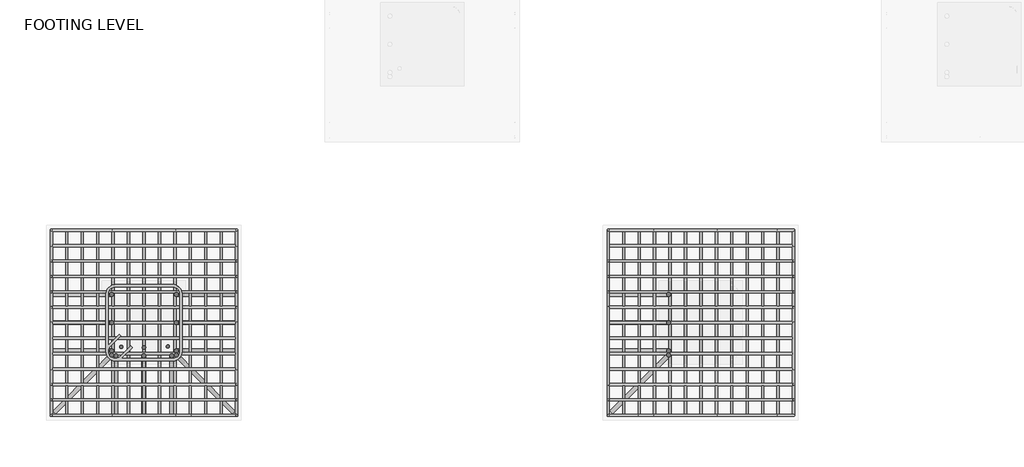
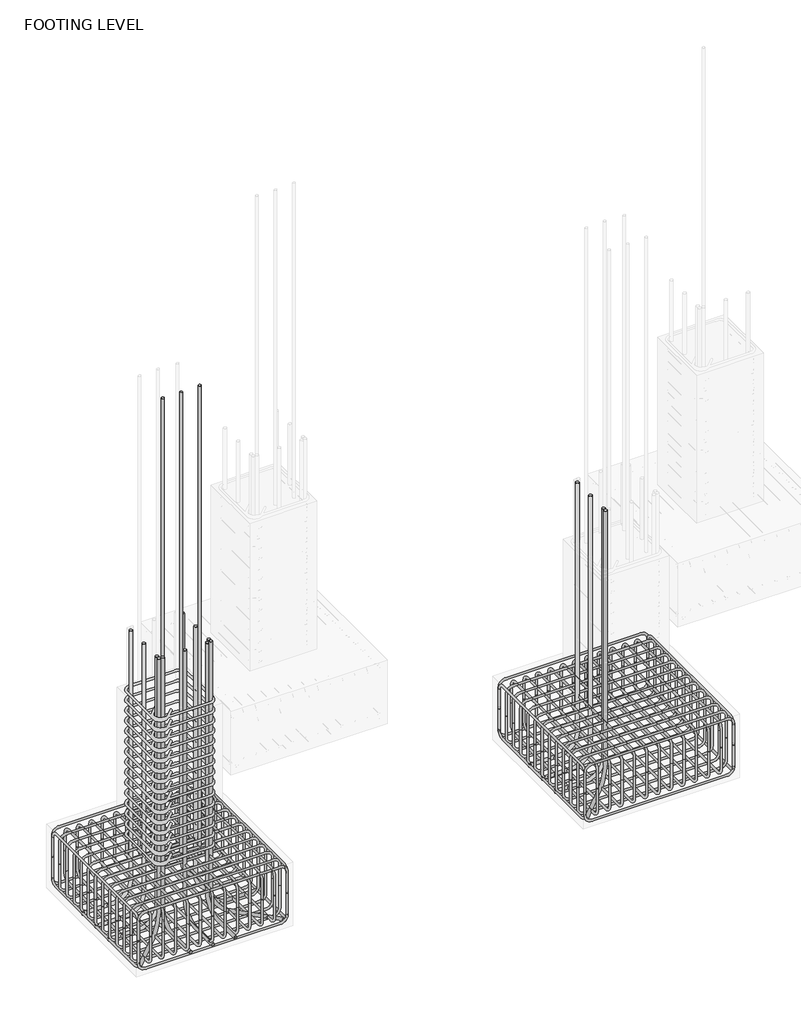
# One storey, part 2 of 10: 20 reinforcing bars.
"""IFC4 building model written with IfcOpenShell, lengths in millimetres."""

from ifc_helpers import new_model, si_unit, point, frame, origin, place, context, project, spatial, polyline, circle_curve, trimmed, segment, composite_curve, source, transform, mapped, element, save
from ifc_brep_helpers import swept_disk

model = new_model("IFC4")

# Units and contexts
model_context = context("Model", 3, world=origin())
ifc_project = project(units=[si_unit("LENGTHUNIT", "METRE", prefix="MILLI")], contexts=[model_context])

# Site, building, storey
site = spatial("IfcSite", under=ifc_project)
building = spatial("IfcBuilding", under=site)
storey = spatial("IfcBuildingStorey", under=building, Name="FOOTING LEVEL", Elevation=-2133.6)

# Reinforcing bars
placement = place(None, origin())
reinforcing_bar_shape = source(origin(), model_context, "Body", "SolidModel", [
    swept_disk(composite_curve([segment(polyline([(-11826.9269037, 756.4829396, -2583.0), (-11826.9269037, 756.4829396, -2905.1)]), True, "CONTINUOUS"), segment(trimmed(circle_curve(frame((-11917.1269037, 756.4829396, -2905.1), z_axis=(0.0, 1.0, 0.0), x_axis=(90.20000000000073, 0.0, 0.0)), 90.2), [point((-11826.9269037, 756.4829396, -2905.1))], [point((-11917.1269037, 756.4829396, -2995.3))], True, "CARTESIAN"), True, "CONTINUOUS"), segment(polyline([(-11917.1269037, 756.4829396, -2995.3), (-13764.9269037, 756.4829396, -2995.3)]), True, "CONTINUOUS"), segment(trimmed(circle_curve(frame((-13764.9269037, 756.4829396, -2905.1), z_axis=(0.0, 1.0, 0.0), x_axis=(0.0, 0.0, -90.20000000000027)), 90.2), [point((-13764.9269037, 756.4829396, -2995.3))], [point((-13855.1269037, 756.4829396, -2905.1))], True, "CARTESIAN"), True, "CONTINUOUS"), segment(polyline([(-13855.1269037, 756.4829396, -2905.1), (-13855.1269037, 756.4829396, -2583.0)]), True, "CONTINUOUS")], self_intersect=False), 12.7),
])
element("IfcReinforcingBar", 1, at=placement, inside=storey, context=model_context, shape_type="MappedRepresentation", body=[
    mapped(reinforcing_bar_shape, transform((0.0, 0.0, 0.0), x_axis=(1.0, 0.0, 0.0), y_axis=(0.0, 1.0, 0.0), z_axis=(0.0, 0.0, 1.0))),
    mapped(reinforcing_bar_shape, transform((0.0, -169.0166667, 0.0), x_axis=(1.0, 0.0, 0.0), y_axis=(0.0, 1.0, 0.0), z_axis=(0.0, 0.0, 1.0))),
    mapped(reinforcing_bar_shape, transform((0.0, -338.0333333, 0.0), x_axis=(1.0, 0.0, 0.0), y_axis=(0.0, 1.0, 0.0), z_axis=(0.0, 0.0, 1.0))),
    mapped(reinforcing_bar_shape, transform((0.0, -507.05, 0.0), x_axis=(1.0, 0.0, 0.0), y_axis=(0.0, 1.0, 0.0), z_axis=(0.0, 0.0, 1.0))),
    mapped(reinforcing_bar_shape, transform((0.0, -676.0666667, 0.0), x_axis=(1.0, 0.0, 0.0), y_axis=(0.0, 1.0, 0.0), z_axis=(0.0, 0.0, 1.0))),
    mapped(reinforcing_bar_shape, transform((0.0, -845.0833333, 0.0), x_axis=(1.0, 0.0, 0.0), y_axis=(0.0, 1.0, 0.0), z_axis=(0.0, 0.0, 1.0))),
    mapped(reinforcing_bar_shape, transform((0.0, -1014.1, 0.0), x_axis=(1.0, 0.0, 0.0), y_axis=(0.0, 1.0, 0.0), z_axis=(0.0, 0.0, 1.0))),
    mapped(reinforcing_bar_shape, transform((0.0, -1183.1166667, 0.0), x_axis=(1.0, 0.0, 0.0), y_axis=(0.0, 1.0, 0.0), z_axis=(0.0, 0.0, 1.0))),
    mapped(reinforcing_bar_shape, transform((0.0, -1352.1333333, 0.0), x_axis=(1.0, 0.0, 0.0), y_axis=(0.0, 1.0, 0.0), z_axis=(0.0, 0.0, 1.0))),
    mapped(reinforcing_bar_shape, transform((0.0, -1521.15, 0.0), x_axis=(1.0, 0.0, 0.0), y_axis=(0.0, 1.0, 0.0), z_axis=(0.0, 0.0, 1.0))),
    mapped(reinforcing_bar_shape, transform((0.0, -1690.1666667, 0.0), x_axis=(1.0, 0.0, 0.0), y_axis=(0.0, 1.0, 0.0), z_axis=(0.0, 0.0, 1.0))),
    mapped(reinforcing_bar_shape, transform((0.0, -1859.1833333, 0.0), x_axis=(1.0, 0.0, 0.0), y_axis=(0.0, 1.0, 0.0), z_axis=(0.0, 0.0, 1.0))),
    mapped(reinforcing_bar_shape, transform((0.0, -2028.2, 0.0), x_axis=(1.0, 0.0, 0.0), y_axis=(0.0, 1.0, 0.0), z_axis=(0.0, 0.0, 1.0))),
])
reinforcing_bar_2_shape = source(origin(), model_context, "Body", "SolidModel", [
    swept_disk(composite_curve([segment(polyline([(-13855.1269037, 756.4829396, -2598.6), (-13855.1269037, 756.4829396, -2276.5)]), True, "CONTINUOUS"), segment(trimmed(circle_curve(frame((-13764.9269037, 756.4829396, -2276.5), z_axis=(0.0, 1.0, 0.0), x_axis=(-90.20000000000073, 0.0, 0.0)), 90.2), [point((-13855.1269037, 756.4829396, -2276.5))], [point((-13764.9269037, 756.4829396, -2186.3))], True, "CARTESIAN"), True, "CONTINUOUS"), segment(polyline([(-13764.9269037, 756.4829396, -2186.3), (-11917.1269037, 756.4829396, -2186.3)]), True, "CONTINUOUS"), segment(trimmed(circle_curve(frame((-11917.1269037, 756.4829396, -2276.5), z_axis=(0.0, 1.0, 0.0), x_axis=(0.0, 0.0, 90.19999999999982)), 90.2), [point((-11917.1269037, 756.4829396, -2186.3))], [point((-11826.9269037, 756.4829396, -2276.5))], True, "CARTESIAN"), True, "CONTINUOUS"), segment(polyline([(-11826.9269037, 756.4829396, -2276.5), (-11826.9269037, 756.4829396, -2598.6)]), True, "CONTINUOUS")], self_intersect=False), 12.7),
])
element("IfcReinforcingBar", 2, at=placement, inside=storey, context=model_context, shape_type="MappedRepresentation", body=[
    mapped(reinforcing_bar_2_shape, transform((0.0, 0.0, 0.0), x_axis=(1.0, 0.0, 0.0), y_axis=(0.0, 1.0, 0.0), z_axis=(0.0, 0.0, 1.0))),
    mapped(reinforcing_bar_2_shape, transform((0.0, -169.0166667, 0.0), x_axis=(1.0, 0.0, 0.0), y_axis=(0.0, 1.0, 0.0), z_axis=(0.0, 0.0, 1.0))),
    mapped(reinforcing_bar_2_shape, transform((0.0, -338.0333333, 0.0), x_axis=(1.0, 0.0, 0.0), y_axis=(0.0, 1.0, 0.0), z_axis=(0.0, 0.0, 1.0))),
    mapped(reinforcing_bar_2_shape, transform((0.0, -507.05, 0.0), x_axis=(1.0, 0.0, 0.0), y_axis=(0.0, 1.0, 0.0), z_axis=(0.0, 0.0, 1.0))),
    mapped(reinforcing_bar_2_shape, transform((0.0, -676.0666667, 0.0), x_axis=(1.0, 0.0, 0.0), y_axis=(0.0, 1.0, 0.0), z_axis=(0.0, 0.0, 1.0))),
    mapped(reinforcing_bar_2_shape, transform((0.0, -845.0833333, 0.0), x_axis=(1.0, 0.0, 0.0), y_axis=(0.0, 1.0, 0.0), z_axis=(0.0, 0.0, 1.0))),
    mapped(reinforcing_bar_2_shape, transform((0.0, -1014.1, 0.0), x_axis=(1.0, 0.0, 0.0), y_axis=(0.0, 1.0, 0.0), z_axis=(0.0, 0.0, 1.0))),
    mapped(reinforcing_bar_2_shape, transform((0.0, -1183.1166667, 0.0), x_axis=(1.0, 0.0, 0.0), y_axis=(0.0, 1.0, 0.0), z_axis=(0.0, 0.0, 1.0))),
    mapped(reinforcing_bar_2_shape, transform((0.0, -1352.1333333, 0.0), x_axis=(1.0, 0.0, 0.0), y_axis=(0.0, 1.0, 0.0), z_axis=(0.0, 0.0, 1.0))),
    mapped(reinforcing_bar_2_shape, transform((0.0, -1521.15, 0.0), x_axis=(1.0, 0.0, 0.0), y_axis=(0.0, 1.0, 0.0), z_axis=(0.0, 0.0, 1.0))),
    mapped(reinforcing_bar_2_shape, transform((0.0, -1690.1666667, 0.0), x_axis=(1.0, 0.0, 0.0), y_axis=(0.0, 1.0, 0.0), z_axis=(0.0, 0.0, 1.0))),
    mapped(reinforcing_bar_2_shape, transform((0.0, -1859.1833333, 0.0), x_axis=(1.0, 0.0, 0.0), y_axis=(0.0, 1.0, 0.0), z_axis=(0.0, 0.0, 1.0))),
    mapped(reinforcing_bar_2_shape, transform((0.0, -2028.2, 0.0), x_axis=(1.0, 0.0, 0.0), y_axis=(0.0, 1.0, 0.0), z_axis=(0.0, 0.0, 1.0))),
])
reinforcing_bar_3_shape = source(origin(), model_context, "Body", "SolidModel", [
    swept_disk(composite_curve([segment(polyline([(-11826.9269037, -1271.7170604, -2559.4978077), (-11826.9269037, -1271.7170604, -2881.5978077)]), True, "CONTINUOUS"), segment(trimmed(circle_curve(frame((-11826.9269037, -1181.5170604, -2881.5978077), z_axis=(1.0, 0.0, 0.0), x_axis=(0.0, -90.20000000000005, 0.0)), 90.2), [point((-11826.9269037, -1271.7170604, -2881.5978077))], [point((-11826.9269037, -1181.5170604, -2971.7978077))], True, "CARTESIAN"), True, "CONTINUOUS"), segment(polyline([(-11826.9269037, -1181.5170604, -2971.7978077), (-11826.9269037, 666.2829396, -2971.7978077)]), True, "CONTINUOUS"), segment(trimmed(circle_curve(frame((-11826.9269037, 666.2829396, -2881.5978077), z_axis=(1.0, 0.0, 0.0), x_axis=(0.0, 0.0, -90.19999999999982)), 90.2), [point((-11826.9269037, 666.2829396, -2971.7978077))], [point((-11826.9269037, 756.4829396, -2881.5978077))], True, "CARTESIAN"), True, "CONTINUOUS"), segment(polyline([(-11826.9269037, 756.4829396, -2881.5978077), (-11826.9269037, 756.4829396, -2559.4978077)]), True, "CONTINUOUS")], self_intersect=False), 12.7),
])
element("IfcReinforcingBar", 3, at=placement, inside=storey, context=model_context, shape_type="MappedRepresentation", body=[
    mapped(reinforcing_bar_3_shape, transform((0.0, 0.0, 0.0), x_axis=(1.0, 0.0, 0.0), y_axis=(0.0, 1.0, 0.0), z_axis=(0.0, 0.0, 1.0))),
    mapped(reinforcing_bar_3_shape, transform((-169.0166667, 0.0, 0.0), x_axis=(1.0, 0.0, 0.0), y_axis=(0.0, 1.0, 0.0), z_axis=(0.0, 0.0, 1.0))),
    mapped(reinforcing_bar_3_shape, transform((-338.0333333, 0.0, 0.0), x_axis=(1.0, 0.0, 0.0), y_axis=(0.0, 1.0, 0.0), z_axis=(0.0, 0.0, 1.0))),
    mapped(reinforcing_bar_3_shape, transform((-507.05, 0.0, 0.0), x_axis=(1.0, 0.0, 0.0), y_axis=(0.0, 1.0, 0.0), z_axis=(0.0, 0.0, 1.0))),
    mapped(reinforcing_bar_3_shape, transform((-676.0666667, 0.0, 0.0), x_axis=(1.0, 0.0, 0.0), y_axis=(0.0, 1.0, 0.0), z_axis=(0.0, 0.0, 1.0))),
    mapped(reinforcing_bar_3_shape, transform((-845.0833333, 0.0, 0.0), x_axis=(1.0, 0.0, 0.0), y_axis=(0.0, 1.0, 0.0), z_axis=(0.0, 0.0, 1.0))),
    mapped(reinforcing_bar_3_shape, transform((-1014.1, 0.0, 0.0), x_axis=(1.0, 0.0, 0.0), y_axis=(0.0, 1.0, 0.0), z_axis=(0.0, 0.0, 1.0))),
    mapped(reinforcing_bar_3_shape, transform((-1183.1166667, 0.0, 0.0), x_axis=(1.0, 0.0, 0.0), y_axis=(0.0, 1.0, 0.0), z_axis=(0.0, 0.0, 1.0))),
    mapped(reinforcing_bar_3_shape, transform((-1352.1333333, 0.0, 0.0), x_axis=(1.0, 0.0, 0.0), y_axis=(0.0, 1.0, 0.0), z_axis=(0.0, 0.0, 1.0))),
    mapped(reinforcing_bar_3_shape, transform((-1521.15, 0.0, 0.0), x_axis=(1.0, 0.0, 0.0), y_axis=(0.0, 1.0, 0.0), z_axis=(0.0, 0.0, 1.0))),
    mapped(reinforcing_bar_3_shape, transform((-1690.1666667, 0.0, 0.0), x_axis=(1.0, 0.0, 0.0), y_axis=(0.0, 1.0, 0.0), z_axis=(0.0, 0.0, 1.0))),
    mapped(reinforcing_bar_3_shape, transform((-1859.1833333, 0.0, 0.0), x_axis=(1.0, 0.0, 0.0), y_axis=(0.0, 1.0, 0.0), z_axis=(0.0, 0.0, 1.0))),
    mapped(reinforcing_bar_3_shape, transform((-2028.2, 0.0, 0.0), x_axis=(1.0, 0.0, 0.0), y_axis=(0.0, 1.0, 0.0), z_axis=(0.0, 0.0, 1.0))),
])
reinforcing_bar_4_shape = source(origin(), model_context, "Body", "SolidModel", [
    swept_disk(composite_curve([segment(polyline([(-13855.1269037, -1271.7170604, -2622.9919875), (-13855.1269037, -1271.7170604, -2300.8919875)]), True, "CONTINUOUS"), segment(trimmed(circle_curve(frame((-13855.1269037, -1181.5170604, -2300.8919875), z_axis=(-1.0, 0.0, 0.0), x_axis=(0.0, -90.20000000000005, 0.0)), 90.2), [point((-13855.1269037, -1271.7170604, -2300.8919875))], [point((-13855.1269037, -1181.5170604, -2210.6919875))], True, "CARTESIAN"), True, "CONTINUOUS"), segment(polyline([(-13855.1269037, -1181.5170604, -2210.6919875), (-13855.1269037, 666.2829396, -2210.6919875)]), True, "CONTINUOUS"), segment(trimmed(circle_curve(frame((-13855.1269037, 666.2829396, -2300.8919875), z_axis=(-1.0, 0.0, 0.0), x_axis=(0.0, 0.0, 90.20000000000027)), 90.2), [point((-13855.1269037, 666.2829396, -2210.6919875))], [point((-13855.1269037, 756.4829396, -2300.8919875))], True, "CARTESIAN"), True, "CONTINUOUS"), segment(polyline([(-13855.1269037, 756.4829396, -2300.8919875), (-13855.1269037, 756.4829396, -2622.9919875)]), True, "CONTINUOUS")], self_intersect=False), 12.7),
])
element("IfcReinforcingBar", 4, at=placement, inside=storey, context=model_context, shape_type="MappedRepresentation", body=[
    mapped(reinforcing_bar_4_shape, transform((0.0, 0.0, 0.0), x_axis=(1.0, 0.0, 0.0), y_axis=(0.0, 1.0, 0.0), z_axis=(0.0, 0.0, 1.0))),
    mapped(reinforcing_bar_4_shape, transform((169.0166667, 0.0, 0.0), x_axis=(1.0, 0.0, 0.0), y_axis=(0.0, 1.0, 0.0), z_axis=(0.0, 0.0, 1.0))),
    mapped(reinforcing_bar_4_shape, transform((338.0333333, 0.0, 0.0), x_axis=(1.0, 0.0, 0.0), y_axis=(0.0, 1.0, 0.0), z_axis=(0.0, 0.0, 1.0))),
    mapped(reinforcing_bar_4_shape, transform((507.05, 0.0, 0.0), x_axis=(1.0, 0.0, 0.0), y_axis=(0.0, 1.0, 0.0), z_axis=(0.0, 0.0, 1.0))),
    mapped(reinforcing_bar_4_shape, transform((676.0666667, 0.0, 0.0), x_axis=(1.0, 0.0, 0.0), y_axis=(0.0, 1.0, 0.0), z_axis=(0.0, 0.0, 1.0))),
    mapped(reinforcing_bar_4_shape, transform((845.0833333, 0.0, 0.0), x_axis=(1.0, 0.0, 0.0), y_axis=(0.0, 1.0, 0.0), z_axis=(0.0, 0.0, 1.0))),
    mapped(reinforcing_bar_4_shape, transform((1014.1, 0.0, 0.0), x_axis=(1.0, 0.0, 0.0), y_axis=(0.0, 1.0, 0.0), z_axis=(0.0, 0.0, 1.0))),
    mapped(reinforcing_bar_4_shape, transform((1183.1166667, 0.0, 0.0), x_axis=(1.0, 0.0, 0.0), y_axis=(0.0, 1.0, 0.0), z_axis=(0.0, 0.0, 1.0))),
    mapped(reinforcing_bar_4_shape, transform((1352.1333333, 0.0, 0.0), x_axis=(1.0, 0.0, 0.0), y_axis=(0.0, 1.0, 0.0), z_axis=(0.0, 0.0, 1.0))),
    mapped(reinforcing_bar_4_shape, transform((1521.15, 0.0, 0.0), x_axis=(1.0, 0.0, 0.0), y_axis=(0.0, 1.0, 0.0), z_axis=(0.0, 0.0, 1.0))),
    mapped(reinforcing_bar_4_shape, transform((1690.1666667, 0.0, 0.0), x_axis=(1.0, 0.0, 0.0), y_axis=(0.0, 1.0, 0.0), z_axis=(0.0, 0.0, 1.0))),
    mapped(reinforcing_bar_4_shape, transform((1859.1833333, 0.0, 0.0), x_axis=(1.0, 0.0, 0.0), y_axis=(0.0, 1.0, 0.0), z_axis=(0.0, 0.0, 1.0))),
    mapped(reinforcing_bar_4_shape, transform((2028.2, 0.0, 0.0), x_axis=(1.0, 0.0, 0.0), y_axis=(0.0, 1.0, 0.0), z_axis=(0.0, 0.0, 1.0))),
])
reinforcing_bar_5_shape = source(origin(), model_context, "Body", "SolidModel", [
    swept_disk(composite_curve([segment(polyline([(-5730.9269037, 756.4829396, -2583.0), (-5730.9269037, 756.4829396, -2905.1)]), True, "CONTINUOUS"), segment(trimmed(circle_curve(frame((-5821.1269037, 756.4829396, -2905.1), z_axis=(0.0, 1.0, 0.0), x_axis=(90.19999999999982, 0.0, 0.0)), 90.2), [point((-5730.9269037, 756.4829396, -2905.1))], [point((-5821.1269037, 756.4829396, -2995.3))], True, "CARTESIAN"), True, "CONTINUOUS"), segment(polyline([(-5821.1269037, 756.4829396, -2995.3), (-7668.9269037, 756.4829396, -2995.3)]), True, "CONTINUOUS"), segment(trimmed(circle_curve(frame((-7668.9269037, 756.4829396, -2905.1), z_axis=(0.0, 1.0, 0.0), x_axis=(0.0, 0.0, -90.20000000000027)), 90.2), [point((-7668.9269037, 756.4829396, -2995.3))], [point((-7759.1269037, 756.4829396, -2905.1))], True, "CARTESIAN"), True, "CONTINUOUS"), segment(polyline([(-7759.1269037, 756.4829396, -2905.1), (-7759.1269037, 756.4829396, -2583.0)]), True, "CONTINUOUS")], self_intersect=False), 12.7),
])
element("IfcReinforcingBar", 5, at=placement, inside=storey, context=model_context, shape_type="MappedRepresentation", body=[
    mapped(reinforcing_bar_5_shape, transform((0.0, 0.0, 0.0), x_axis=(1.0, 0.0, 0.0), y_axis=(0.0, 1.0, 0.0), z_axis=(0.0, 0.0, 1.0))),
    mapped(reinforcing_bar_5_shape, transform((0.0, -169.0166667, 0.0), x_axis=(1.0, 0.0, 0.0), y_axis=(0.0, 1.0, 0.0), z_axis=(0.0, 0.0, 1.0))),
    mapped(reinforcing_bar_5_shape, transform((0.0, -338.0333333, 0.0), x_axis=(1.0, 0.0, 0.0), y_axis=(0.0, 1.0, 0.0), z_axis=(0.0, 0.0, 1.0))),
    mapped(reinforcing_bar_5_shape, transform((0.0, -507.05, 0.0), x_axis=(1.0, 0.0, 0.0), y_axis=(0.0, 1.0, 0.0), z_axis=(0.0, 0.0, 1.0))),
    mapped(reinforcing_bar_5_shape, transform((0.0, -676.0666667, 0.0), x_axis=(1.0, 0.0, 0.0), y_axis=(0.0, 1.0, 0.0), z_axis=(0.0, 0.0, 1.0))),
    mapped(reinforcing_bar_5_shape, transform((0.0, -845.0833333, 0.0), x_axis=(1.0, 0.0, 0.0), y_axis=(0.0, 1.0, 0.0), z_axis=(0.0, 0.0, 1.0))),
    mapped(reinforcing_bar_5_shape, transform((0.0, -1014.1, 0.0), x_axis=(1.0, 0.0, 0.0), y_axis=(0.0, 1.0, 0.0), z_axis=(0.0, 0.0, 1.0))),
    mapped(reinforcing_bar_5_shape, transform((0.0, -1183.1166667, 0.0), x_axis=(1.0, 0.0, 0.0), y_axis=(0.0, 1.0, 0.0), z_axis=(0.0, 0.0, 1.0))),
    mapped(reinforcing_bar_5_shape, transform((0.0, -1352.1333333, 0.0), x_axis=(1.0, 0.0, 0.0), y_axis=(0.0, 1.0, 0.0), z_axis=(0.0, 0.0, 1.0))),
    mapped(reinforcing_bar_5_shape, transform((0.0, -1521.15, 0.0), x_axis=(1.0, 0.0, 0.0), y_axis=(0.0, 1.0, 0.0), z_axis=(0.0, 0.0, 1.0))),
    mapped(reinforcing_bar_5_shape, transform((0.0, -1690.1666667, 0.0), x_axis=(1.0, 0.0, 0.0), y_axis=(0.0, 1.0, 0.0), z_axis=(0.0, 0.0, 1.0))),
    mapped(reinforcing_bar_5_shape, transform((0.0, -1859.1833333, 0.0), x_axis=(1.0, 0.0, 0.0), y_axis=(0.0, 1.0, 0.0), z_axis=(0.0, 0.0, 1.0))),
    mapped(reinforcing_bar_5_shape, transform((0.0, -2028.2, 0.0), x_axis=(1.0, 0.0, 0.0), y_axis=(0.0, 1.0, 0.0), z_axis=(0.0, 0.0, 1.0))),
])
reinforcing_bar_6_shape = source(origin(), model_context, "Body", "SolidModel", [
    swept_disk(composite_curve([segment(polyline([(-7759.1269037, 756.4829396, -2598.6), (-7759.1269037, 756.4829396, -2276.5)]), True, "CONTINUOUS"), segment(trimmed(circle_curve(frame((-7668.9269037, 756.4829396, -2276.5), z_axis=(0.0, 1.0, 0.0), x_axis=(-90.19999999999982, 0.0, 0.0)), 90.2), [point((-7759.1269037, 756.4829396, -2276.5))], [point((-7668.9269037, 756.4829396, -2186.3))], True, "CARTESIAN"), True, "CONTINUOUS"), segment(polyline([(-7668.9269037, 756.4829396, -2186.3), (-5821.1269037, 756.4829396, -2186.3)]), True, "CONTINUOUS"), segment(trimmed(circle_curve(frame((-5821.1269037, 756.4829396, -2276.5), z_axis=(0.0, 1.0, 0.0), x_axis=(0.0, 0.0, 90.19999999999982)), 90.2), [point((-5821.1269037, 756.4829396, -2186.3))], [point((-5730.9269037, 756.4829396, -2276.5))], True, "CARTESIAN"), True, "CONTINUOUS"), segment(polyline([(-5730.9269037, 756.4829396, -2276.5), (-5730.9269037, 756.4829396, -2598.6)]), True, "CONTINUOUS")], self_intersect=False), 12.7),
])
element("IfcReinforcingBar", 6, at=placement, inside=storey, context=model_context, shape_type="MappedRepresentation", body=[
    mapped(reinforcing_bar_6_shape, transform((0.0, 0.0, 0.0), x_axis=(1.0, 0.0, 0.0), y_axis=(0.0, 1.0, 0.0), z_axis=(0.0, 0.0, 1.0))),
    mapped(reinforcing_bar_6_shape, transform((0.0, -169.0166667, 0.0), x_axis=(1.0, 0.0, 0.0), y_axis=(0.0, 1.0, 0.0), z_axis=(0.0, 0.0, 1.0))),
    mapped(reinforcing_bar_6_shape, transform((0.0, -338.0333333, 0.0), x_axis=(1.0, 0.0, 0.0), y_axis=(0.0, 1.0, 0.0), z_axis=(0.0, 0.0, 1.0))),
    mapped(reinforcing_bar_6_shape, transform((0.0, -507.05, 0.0), x_axis=(1.0, 0.0, 0.0), y_axis=(0.0, 1.0, 0.0), z_axis=(0.0, 0.0, 1.0))),
    mapped(reinforcing_bar_6_shape, transform((0.0, -676.0666667, 0.0), x_axis=(1.0, 0.0, 0.0), y_axis=(0.0, 1.0, 0.0), z_axis=(0.0, 0.0, 1.0))),
    mapped(reinforcing_bar_6_shape, transform((0.0, -845.0833333, 0.0), x_axis=(1.0, 0.0, 0.0), y_axis=(0.0, 1.0, 0.0), z_axis=(0.0, 0.0, 1.0))),
    mapped(reinforcing_bar_6_shape, transform((0.0, -1014.1, 0.0), x_axis=(1.0, 0.0, 0.0), y_axis=(0.0, 1.0, 0.0), z_axis=(0.0, 0.0, 1.0))),
    mapped(reinforcing_bar_6_shape, transform((0.0, -1183.1166667, 0.0), x_axis=(1.0, 0.0, 0.0), y_axis=(0.0, 1.0, 0.0), z_axis=(0.0, 0.0, 1.0))),
    mapped(reinforcing_bar_6_shape, transform((0.0, -1352.1333333, 0.0), x_axis=(1.0, 0.0, 0.0), y_axis=(0.0, 1.0, 0.0), z_axis=(0.0, 0.0, 1.0))),
    mapped(reinforcing_bar_6_shape, transform((0.0, -1521.15, 0.0), x_axis=(1.0, 0.0, 0.0), y_axis=(0.0, 1.0, 0.0), z_axis=(0.0, 0.0, 1.0))),
    mapped(reinforcing_bar_6_shape, transform((0.0, -1690.1666667, 0.0), x_axis=(1.0, 0.0, 0.0), y_axis=(0.0, 1.0, 0.0), z_axis=(0.0, 0.0, 1.0))),
    mapped(reinforcing_bar_6_shape, transform((0.0, -1859.1833333, 0.0), x_axis=(1.0, 0.0, 0.0), y_axis=(0.0, 1.0, 0.0), z_axis=(0.0, 0.0, 1.0))),
    mapped(reinforcing_bar_6_shape, transform((0.0, -2028.2, 0.0), x_axis=(1.0, 0.0, 0.0), y_axis=(0.0, 1.0, 0.0), z_axis=(0.0, 0.0, 1.0))),
])
reinforcing_bar_7_shape = source(origin(), model_context, "Body", "SolidModel", [
    swept_disk(composite_curve([segment(polyline([(-5730.9269037, -1271.7170604, -2559.4978077), (-5730.9269037, -1271.7170604, -2881.5978077)]), True, "CONTINUOUS"), segment(trimmed(circle_curve(frame((-5730.9269037, -1181.5170604, -2881.5978077), z_axis=(1.0, 0.0, 0.0), x_axis=(0.0, -90.20000000000005, 0.0)), 90.2), [point((-5730.9269037, -1271.7170604, -2881.5978077))], [point((-5730.9269037, -1181.5170604, -2971.7978077))], True, "CARTESIAN"), True, "CONTINUOUS"), segment(polyline([(-5730.9269037, -1181.5170604, -2971.7978077), (-5730.9269037, 666.2829396, -2971.7978077)]), True, "CONTINUOUS"), segment(trimmed(circle_curve(frame((-5730.9269037, 666.2829396, -2881.5978077), z_axis=(1.0, 0.0, 0.0), x_axis=(0.0, 0.0, -90.19999999999982)), 90.2), [point((-5730.9269037, 666.2829396, -2971.7978077))], [point((-5730.9269037, 756.4829396, -2881.5978077))], True, "CARTESIAN"), True, "CONTINUOUS"), segment(polyline([(-5730.9269037, 756.4829396, -2881.5978077), (-5730.9269037, 756.4829396, -2559.4978077)]), True, "CONTINUOUS")], self_intersect=False), 12.7),
])
element("IfcReinforcingBar", 7, at=placement, inside=storey, context=model_context, shape_type="MappedRepresentation", body=[
    mapped(reinforcing_bar_7_shape, transform((0.0, 0.0, 0.0), x_axis=(1.0, 0.0, 0.0), y_axis=(0.0, 1.0, 0.0), z_axis=(0.0, 0.0, 1.0))),
    mapped(reinforcing_bar_7_shape, transform((-169.0166667, 0.0, 0.0), x_axis=(1.0, 0.0, 0.0), y_axis=(0.0, 1.0, 0.0), z_axis=(0.0, 0.0, 1.0))),
    mapped(reinforcing_bar_7_shape, transform((-338.0333333, 0.0, 0.0), x_axis=(1.0, 0.0, 0.0), y_axis=(0.0, 1.0, 0.0), z_axis=(0.0, 0.0, 1.0))),
    mapped(reinforcing_bar_7_shape, transform((-507.05, 0.0, 0.0), x_axis=(1.0, 0.0, 0.0), y_axis=(0.0, 1.0, 0.0), z_axis=(0.0, 0.0, 1.0))),
    mapped(reinforcing_bar_7_shape, transform((-676.0666667, 0.0, 0.0), x_axis=(1.0, 0.0, 0.0), y_axis=(0.0, 1.0, 0.0), z_axis=(0.0, 0.0, 1.0))),
    mapped(reinforcing_bar_7_shape, transform((-845.0833333, 0.0, 0.0), x_axis=(1.0, 0.0, 0.0), y_axis=(0.0, 1.0, 0.0), z_axis=(0.0, 0.0, 1.0))),
    mapped(reinforcing_bar_7_shape, transform((-1014.1, 0.0, 0.0), x_axis=(1.0, 0.0, 0.0), y_axis=(0.0, 1.0, 0.0), z_axis=(0.0, 0.0, 1.0))),
    mapped(reinforcing_bar_7_shape, transform((-1183.1166667, 0.0, 0.0), x_axis=(1.0, 0.0, 0.0), y_axis=(0.0, 1.0, 0.0), z_axis=(0.0, 0.0, 1.0))),
    mapped(reinforcing_bar_7_shape, transform((-1352.1333333, 0.0, 0.0), x_axis=(1.0, 0.0, 0.0), y_axis=(0.0, 1.0, 0.0), z_axis=(0.0, 0.0, 1.0))),
    mapped(reinforcing_bar_7_shape, transform((-1521.15, 0.0, 0.0), x_axis=(1.0, 0.0, 0.0), y_axis=(0.0, 1.0, 0.0), z_axis=(0.0, 0.0, 1.0))),
    mapped(reinforcing_bar_7_shape, transform((-1690.1666667, 0.0, 0.0), x_axis=(1.0, 0.0, 0.0), y_axis=(0.0, 1.0, 0.0), z_axis=(0.0, 0.0, 1.0))),
    mapped(reinforcing_bar_7_shape, transform((-1859.1833333, 0.0, 0.0), x_axis=(1.0, 0.0, 0.0), y_axis=(0.0, 1.0, 0.0), z_axis=(0.0, 0.0, 1.0))),
    mapped(reinforcing_bar_7_shape, transform((-2028.2, 0.0, 0.0), x_axis=(1.0, 0.0, 0.0), y_axis=(0.0, 1.0, 0.0), z_axis=(0.0, 0.0, 1.0))),
])
reinforcing_bar_8_shape = source(origin(), model_context, "Body", "SolidModel", [
    swept_disk(composite_curve([segment(polyline([(-7759.1269037, -1271.7170604, -2622.9919875), (-7759.1269037, -1271.7170604, -2300.8919875)]), True, "CONTINUOUS"), segment(trimmed(circle_curve(frame((-7759.1269037, -1181.5170604, -2300.8919875), z_axis=(-1.0, 0.0, 0.0), x_axis=(0.0, -90.20000000000005, 0.0)), 90.2), [point((-7759.1269037, -1271.7170604, -2300.8919875))], [point((-7759.1269037, -1181.5170604, -2210.6919875))], True, "CARTESIAN"), True, "CONTINUOUS"), segment(polyline([(-7759.1269037, -1181.5170604, -2210.6919875), (-7759.1269037, 666.2829396, -2210.6919875)]), True, "CONTINUOUS"), segment(trimmed(circle_curve(frame((-7759.1269037, 666.2829396, -2300.8919875), z_axis=(-1.0, 0.0, 0.0), x_axis=(0.0, 0.0, 90.20000000000027)), 90.2), [point((-7759.1269037, 666.2829396, -2210.6919875))], [point((-7759.1269037, 756.4829396, -2300.8919875))], True, "CARTESIAN"), True, "CONTINUOUS"), segment(polyline([(-7759.1269037, 756.4829396, -2300.8919875), (-7759.1269037, 756.4829396, -2622.9919875)]), True, "CONTINUOUS")], self_intersect=False), 12.7),
])
element("IfcReinforcingBar", 8, at=placement, inside=storey, context=model_context, shape_type="MappedRepresentation", body=[
    mapped(reinforcing_bar_8_shape, transform((0.0, 0.0, 0.0), x_axis=(1.0, 0.0, 0.0), y_axis=(0.0, 1.0, 0.0), z_axis=(0.0, 0.0, 1.0))),
    mapped(reinforcing_bar_8_shape, transform((169.0166667, 0.0, 0.0), x_axis=(1.0, 0.0, 0.0), y_axis=(0.0, 1.0, 0.0), z_axis=(0.0, 0.0, 1.0))),
    mapped(reinforcing_bar_8_shape, transform((338.0333333, 0.0, 0.0), x_axis=(1.0, 0.0, 0.0), y_axis=(0.0, 1.0, 0.0), z_axis=(0.0, 0.0, 1.0))),
    mapped(reinforcing_bar_8_shape, transform((507.05, 0.0, 0.0), x_axis=(1.0, 0.0, 0.0), y_axis=(0.0, 1.0, 0.0), z_axis=(0.0, 0.0, 1.0))),
    mapped(reinforcing_bar_8_shape, transform((676.0666667, 0.0, 0.0), x_axis=(1.0, 0.0, 0.0), y_axis=(0.0, 1.0, 0.0), z_axis=(0.0, 0.0, 1.0))),
    mapped(reinforcing_bar_8_shape, transform((845.0833333, 0.0, 0.0), x_axis=(1.0, 0.0, 0.0), y_axis=(0.0, 1.0, 0.0), z_axis=(0.0, 0.0, 1.0))),
    mapped(reinforcing_bar_8_shape, transform((1014.1, 0.0, 0.0), x_axis=(1.0, 0.0, 0.0), y_axis=(0.0, 1.0, 0.0), z_axis=(0.0, 0.0, 1.0))),
    mapped(reinforcing_bar_8_shape, transform((1183.1166667, 0.0, 0.0), x_axis=(1.0, 0.0, 0.0), y_axis=(0.0, 1.0, 0.0), z_axis=(0.0, 0.0, 1.0))),
    mapped(reinforcing_bar_8_shape, transform((1352.1333333, 0.0, 0.0), x_axis=(1.0, 0.0, 0.0), y_axis=(0.0, 1.0, 0.0), z_axis=(0.0, 0.0, 1.0))),
    mapped(reinforcing_bar_8_shape, transform((1521.15, 0.0, 0.0), x_axis=(1.0, 0.0, 0.0), y_axis=(0.0, 1.0, 0.0), z_axis=(0.0, 0.0, 1.0))),
    mapped(reinforcing_bar_8_shape, transform((1690.1666667, 0.0, 0.0), x_axis=(1.0, 0.0, 0.0), y_axis=(0.0, 1.0, 0.0), z_axis=(0.0, 0.0, 1.0))),
    mapped(reinforcing_bar_8_shape, transform((1859.1833333, 0.0, 0.0), x_axis=(1.0, 0.0, 0.0), y_axis=(0.0, 1.0, 0.0), z_axis=(0.0, 0.0, 1.0))),
    mapped(reinforcing_bar_8_shape, transform((2028.2, 0.0, 0.0), x_axis=(1.0, 0.0, 0.0), y_axis=(0.0, 1.0, 0.0), z_axis=(0.0, 0.0, 1.0))),
])
reinforcing_bar_9_shape = source(origin(), model_context, "Body", "SolidModel", [
    swept_disk(composite_curve([segment(polyline([(-12978.1462687, -522.2984887, 0.0), (-13091.545872, -635.6980921, 0.0)]), True, "CONTINUOUS"), segment(trimmed(circle_curve(frame((-13155.3269037, -571.9170604, 0.0), z_axis=(0.0, 0.0, -1.0), x_axis=(63.78103169999849, -63.781031700000085, 0.0)), 90.2), [point((-13091.545872, -635.6980921, 0.0))], [point((-13245.5269037, -571.9170604, 0.0))], True, "CARTESIAN"), True, "CONTINUOUS"), segment(polyline([(-13245.5269037, -571.9170604, 0.0), (-13245.5269037, 56.6829396, 0.0)]), True, "CONTINUOUS"), segment(trimmed(circle_curve(frame((-13155.3269037, 56.6829396, 0.0), z_axis=(0.0, 0.0, -1.0), x_axis=(-90.20000000000073, 0.0, 0.0)), 90.2), [point((-13245.5269037, 56.6829396, 0.0))], [point((-13155.3269037, 146.8829396, 0.0))], True, "CARTESIAN"), True, "CONTINUOUS"), segment(polyline([(-13155.3269037, 146.8829396, 0.0), (-12526.7269037, 146.8829396, 0.0)]), True, "CONTINUOUS"), segment(trimmed(circle_curve(frame((-12526.7269037, 56.7273645, 2.8305953), z_axis=(0.0, -0.03138132276777647, -0.9995074850051623), x_axis=(0.0, 90.1555751, -2.8305953)), 90.2), [point((-12526.7269037, 146.8829396, 0.0))], [point((-12436.5269037, 56.7273645, 2.8305953))], True, "CARTESIAN"), True, "CONTINUOUS"), segment(polyline([(-12436.5269037, 56.7273645, 2.8305953), (-12436.5269037, -571.9614853, 22.5694047)]), True, "CONTINUOUS"), segment(trimmed(circle_curve(frame((-12526.7269037, -571.9614853, 22.5694047), z_axis=(0.0, -0.03138132276777647, -0.9995074850051623), x_axis=(90.20000000000073, 0.0, 0.0)), 90.2), [point((-12436.5269037, -571.9614853, 22.5694047))], [point((-12526.7269037, -662.1170604, 25.4))], True, "CARTESIAN"), True, "CONTINUOUS"), segment(polyline([(-12526.7269037, -662.1170604, 25.4), (-13155.3269037, -662.1170604, 25.4)]), True, "CONTINUOUS"), segment(trimmed(circle_curve(frame((-13155.3269037, -571.9170604, 25.4), z_axis=(0.0, 0.0, -1.0), x_axis=(0.0, -90.20000000000005, 0.0)), 90.2), [point((-13155.3269037, -662.1170604, 25.4))], [point((-13219.1079353, -508.1360287, 25.4))], True, "CARTESIAN"), True, "CONTINUOUS"), segment(polyline([(-13219.1079353, -508.1360287, 25.4), (-13105.708332, -394.7364254, 25.4)]), True, "CONTINUOUS")], self_intersect=False), 12.7),
])
element("IfcReinforcingBar", 9, at=placement, inside=storey, context=model_context, shape_type="MappedRepresentation", body=[
    mapped(reinforcing_bar_9_shape, transform((0.0, 0.0, 0.0), x_axis=(1.0, 0.0, 0.0), y_axis=(0.0, 1.0, 0.0), z_axis=(0.0, 0.0, 1.0))),
    mapped(reinforcing_bar_9_shape, transform((0.0, 0.0, -148.6357143), x_axis=(1.0, 0.0, 0.0), y_axis=(0.0, 1.0, 0.0), z_axis=(0.0, 0.0, 1.0))),
    mapped(reinforcing_bar_9_shape, transform((0.0, 0.0, -297.2714286), x_axis=(1.0, 0.0, 0.0), y_axis=(0.0, 1.0, 0.0), z_axis=(0.0, 0.0, 1.0))),
    mapped(reinforcing_bar_9_shape, transform((0.0, 0.0, -445.9071429), x_axis=(1.0, 0.0, 0.0), y_axis=(0.0, 1.0, 0.0), z_axis=(0.0, 0.0, 1.0))),
    mapped(reinforcing_bar_9_shape, transform((0.0, 0.0, -594.5428571), x_axis=(1.0, 0.0, 0.0), y_axis=(0.0, 1.0, 0.0), z_axis=(0.0, 0.0, 1.0))),
    mapped(reinforcing_bar_9_shape, transform((0.0, 0.0, -743.1785714), x_axis=(1.0, 0.0, 0.0), y_axis=(0.0, 1.0, 0.0), z_axis=(0.0, 0.0, 1.0))),
    mapped(reinforcing_bar_9_shape, transform((0.0, 0.0, -891.8142857), x_axis=(1.0, 0.0, 0.0), y_axis=(0.0, 1.0, 0.0), z_axis=(0.0, 0.0, 1.0))),
    mapped(reinforcing_bar_9_shape, transform((0.0, 0.0, -1040.45), x_axis=(1.0, 0.0, 0.0), y_axis=(0.0, 1.0, 0.0), z_axis=(0.0, 0.0, 1.0))),
    mapped(reinforcing_bar_9_shape, transform((0.0, 0.0, -1189.0857143), x_axis=(1.0, 0.0, 0.0), y_axis=(0.0, 1.0, 0.0), z_axis=(0.0, 0.0, 1.0))),
    mapped(reinforcing_bar_9_shape, transform((0.0, 0.0, -1337.7214286), x_axis=(1.0, 0.0, 0.0), y_axis=(0.0, 1.0, 0.0), z_axis=(0.0, 0.0, 1.0))),
    mapped(reinforcing_bar_9_shape, transform((0.0, 0.0, -1486.3571429), x_axis=(1.0, 0.0, 0.0), y_axis=(0.0, 1.0, 0.0), z_axis=(0.0, 0.0, 1.0))),
    mapped(reinforcing_bar_9_shape, transform((0.0, 0.0, -1634.9928571), x_axis=(1.0, 0.0, 0.0), y_axis=(0.0, 1.0, 0.0), z_axis=(0.0, 0.0, 1.0))),
    mapped(reinforcing_bar_9_shape, transform((0.0, 0.0, -1783.6285714), x_axis=(1.0, 0.0, 0.0), y_axis=(0.0, 1.0, 0.0), z_axis=(0.0, 0.0, 1.0))),
    mapped(reinforcing_bar_9_shape, transform((0.0, 0.0, -1932.2642857), x_axis=(1.0, 0.0, 0.0), y_axis=(0.0, 1.0, 0.0), z_axis=(0.0, 0.0, 1.0))),
    mapped(reinforcing_bar_9_shape, transform((0.0, 0.0, -2080.9), x_axis=(1.0, 0.0, 0.0), y_axis=(0.0, 1.0, 0.0), z_axis=(0.0, 0.0, 1.0))),
])
element("IfcReinforcingBar", 10, at=placement, inside=storey, context=model_context, shape_type="SolidModel", body=[
    swept_disk(composite_curve([segment(polyline([(-7725.4807966, -1238.0709533, -2976.5), (-7278.5300058, -791.1201626, -2976.5)]), True, "CONTINUOUS"), segment(trimmed(circle_curve(frame((-7278.5300058, -791.1201626, -2722.5), z_axis=(0.7071067811865475, -0.7071067811865477, 0.0), x_axis=(0.0, 0.0, -254.0)), 254.0), [point((-7278.5300058, -791.1201626, -2976.5))], [point((-7098.9248834, -611.5150401, -2722.5))], True, "CARTESIAN"), True, "CONTINUOUS"), segment(polyline([(-7098.9248834, -611.5150401, -2722.5), (-7098.9248834, -611.5150401, 874.4)]), True, "CONTINUOUS")], self_intersect=False), 21.5),
])
reinforcing_bar_10_shape = source(origin(), model_context, "Body", "SolidModel", [
    swept_disk(composite_curve([segment(polyline([(-7761.8269037, -565.9980034, -2976.5), (-7352.9248834, -565.9980034, -2976.5)]), True, "CONTINUOUS"), segment(trimmed(circle_curve(frame((-7352.9248834, -565.9980034, -2722.5), z_axis=(0.0, -1.0, 0.0), x_axis=(0.0, 0.0, -254.0)), 254.0), [point((-7352.9248834, -565.9980034, -2976.5))], [point((-7098.9248834, -565.9980034, -2722.5))], True, "CARTESIAN"), True, "CONTINUOUS"), segment(polyline([(-7098.9248834, -565.9980034, -2722.5), (-7098.9248834, -565.9980034, 874.4)]), True, "CONTINUOUS")], self_intersect=False), 21.5),
])
element("IfcReinforcingBar", 11, at=placement, inside=storey, context=model_context, shape_type="MappedRepresentation", body=[
    mapped(reinforcing_bar_10_shape, transform((0.0, 0.0, 0.0), x_axis=(1.0, 0.0, 0.0), y_axis=(0.0, 1.0, 0.0), z_axis=(0.0, 0.0, 1.0))),
    mapped(reinforcing_bar_10_shape, transform((0.0, 309.128507, 0.0), x_axis=(1.0, 0.0, 0.0), y_axis=(0.0, 1.0, 0.0), z_axis=(0.0, 0.0, 1.0))),
    mapped(reinforcing_bar_10_shape, transform((0.0, 618.2570139, 0.0), x_axis=(1.0, 0.0, 0.0), y_axis=(0.0, 1.0, 0.0), z_axis=(0.0, 0.0, 1.0))),
])
element("IfcReinforcingBar", 12, at=placement, inside=storey, context=model_context, shape_type="SolidModel", body=[
    swept_disk(composite_curve([segment(polyline([(-11860.5730107, -1238.0709533, -2976.5), (-12307.5238015, -791.1201626, -2976.5)]), True, "CONTINUOUS"), segment(trimmed(circle_curve(frame((-12307.5238015, -791.1201626, -2722.5), z_axis=(0.7071067811865508, 0.7071067811865444, 0.0), x_axis=(0.0, 0.0, -254.0)), 254.0), [point((-12307.5238015, -791.1201626, -2976.5))], [point((-12487.1289239, -611.5150401, -2722.5))], True, "CARTESIAN"), True, "CONTINUOUS"), segment(polyline([(-12487.1289239, -611.5150401, -2722.5), (-12487.1289239, -611.5150401, 874.4)]), True, "CONTINUOUS")], self_intersect=False), 21.5),
])
element("IfcReinforcingBar", 13, at=placement, inside=storey, context=model_context, shape_type="SolidModel", body=[
    swept_disk(composite_curve([segment(polyline([(-13821.4807966, -1238.0709533, -2976.5), (-13374.5300058, -791.1201626, -2976.5)]), True, "CONTINUOUS"), segment(trimmed(circle_curve(frame((-13374.5300058, -791.1201626, -2722.5), z_axis=(0.7071067811865475, -0.7071067811865477, 0.0), x_axis=(0.0, 0.0, -254.0)), 254.0), [point((-13374.5300058, -791.1201626, -2976.5))], [point((-13194.9248834, -611.5150401, -2722.5))], True, "CARTESIAN"), True, "CONTINUOUS"), segment(polyline([(-13194.9248834, -611.5150401, -2722.5), (-13194.9248834, -611.5150401, 874.4)]), True, "CONTINUOUS")], self_intersect=False), 21.5),
])
element("IfcReinforcingBar", 14, at=placement, inside=storey, context=model_context, shape_type="SolidModel", body=[
    swept_disk(composite_curve([segment(polyline([(-11860.5730107, -1238.0709533, -2976.5), (-12307.5238015, -791.1201626, -2976.5)]), True, "CONTINUOUS"), segment(trimmed(circle_curve(frame((-12307.5238015, -791.1201626, -2722.5), z_axis=(0.7071067811865508, 0.7071067811865444, 0.0), x_axis=(0.0, 0.0, -254.0)), 254.0), [point((-12307.5238015, -791.1201626, -2976.5))], [point((-12487.1289239, -611.5150401, -2722.5))], True, "CARTESIAN"), True, "CONTINUOUS"), segment(polyline([(-12487.1289239, -611.5150401, -2722.5), (-12487.1289239, -611.5150401, 874.4)]), True, "CONTINUOUS")], self_intersect=False), 21.5),
])
reinforcing_bar_11_shape = source(origin(), model_context, "Body", "SolidModel", [
    swept_disk(composite_curve([segment(polyline([(-11824.2269037, -565.9980034, -2976.5), (-12233.1289239, -565.9980034, -2976.5)]), True, "CONTINUOUS"), segment(trimmed(circle_curve(frame((-12233.1289239, -565.9980034, -2722.5), z_axis=(0.0, 1.0, 0.0), x_axis=(0.0, 0.0, -254.0)), 254.0), [point((-12233.1289239, -565.9980034, -2976.5))], [point((-12487.1289239, -565.9980034, -2722.5))], True, "CARTESIAN"), True, "CONTINUOUS"), segment(polyline([(-12487.1289239, -565.9980034, -2722.5), (-12487.1289239, -565.9980034, 874.4)]), True, "CONTINUOUS")], self_intersect=False), 21.5),
])
element("IfcReinforcingBar", 15, at=placement, inside=storey, context=model_context, shape_type="MappedRepresentation", body=[
    mapped(reinforcing_bar_11_shape, transform((0.0, 0.0, 0.0), x_axis=(1.0, 0.0, 0.0), y_axis=(0.0, 1.0, 0.0), z_axis=(0.0, 0.0, 1.0))),
    mapped(reinforcing_bar_11_shape, transform((0.0, 309.128507, 0.0), x_axis=(1.0, 0.0, 0.0), y_axis=(0.0, 1.0, 0.0), z_axis=(0.0, 0.0, 1.0))),
    mapped(reinforcing_bar_11_shape, transform((0.0, 618.2570139, 0.0), x_axis=(1.0, 0.0, 0.0), y_axis=(0.0, 1.0, 0.0), z_axis=(0.0, 0.0, 1.0))),
])
reinforcing_bar_12_shape = source(origin(), model_context, "Body", "SolidModel", [
    swept_disk(composite_curve([segment(polyline([(-13857.8269037, -565.9980034, -2976.5), (-13448.9248834, -565.9980034, -2976.5)]), True, "CONTINUOUS"), segment(trimmed(circle_curve(frame((-13448.9248834, -565.9980034, -2722.5), z_axis=(0.0, -1.0, 0.0), x_axis=(0.0, 0.0, -254.0)), 254.0), [point((-13448.9248834, -565.9980034, -2976.5))], [point((-13194.9248834, -565.9980034, -2722.5))], True, "CARTESIAN"), True, "CONTINUOUS"), segment(polyline([(-13194.9248834, -565.9980034, -2722.5), (-13194.9248834, -565.9980034, 874.4)]), True, "CONTINUOUS")], self_intersect=False), 21.5),
])
element("IfcReinforcingBar", 16, at=placement, inside=storey, context=model_context, shape_type="MappedRepresentation", body=[
    mapped(reinforcing_bar_12_shape, transform((0.0, 0.0, 0.0), x_axis=(1.0, 0.0, 0.0), y_axis=(0.0, 1.0, 0.0), z_axis=(0.0, 0.0, 1.0))),
    mapped(reinforcing_bar_12_shape, transform((0.0, 309.128507, 0.0), x_axis=(1.0, 0.0, 0.0), y_axis=(0.0, 1.0, 0.0), z_axis=(0.0, 0.0, 1.0))),
    mapped(reinforcing_bar_12_shape, transform((0.0, 618.2570139, 0.0), x_axis=(1.0, 0.0, 0.0), y_axis=(0.0, 1.0, 0.0), z_axis=(0.0, 0.0, 1.0))),
])
reinforcing_bar_13_shape = source(origin(), model_context, "Body", "SolidModel", [
    swept_disk(composite_curve([segment(polyline([(-12537.6587573, -1282.6598713, -2976.5), (-12537.6587573, -873.757851, -2976.5)]), True, "CONTINUOUS"), segment(trimmed(circle_curve(frame((-12537.6587573, -873.757851, -2722.5), z_axis=(1.0, 0.0, 0.0), x_axis=(0.0, 0.0, -254.0)), 254.0), [point((-12537.6587573, -873.757851, -2976.5))], [point((-12537.6587573, -619.757851, -2722.5))], True, "CARTESIAN"), True, "CONTINUOUS"), segment(polyline([(-12537.6587573, -619.757851, -2722.5), (-12537.6587573, -619.757851, 874.4)]), True, "CONTINUOUS")], self_intersect=False), 21.5),
])
element("IfcReinforcingBar", 17, at=placement, inside=storey, context=model_context, shape_type="MappedRepresentation", body=[
    mapped(reinforcing_bar_13_shape, transform((0.0, 0.0, 0.0), x_axis=(1.0, 0.0, 0.0), y_axis=(0.0, 1.0, 0.0), z_axis=(0.0, 0.0, 1.0))),
    mapped(reinforcing_bar_13_shape, transform((-304.9765997, 0.0, 0.0), x_axis=(1.0, 0.0, 0.0), y_axis=(0.0, 1.0, 0.0), z_axis=(0.0, 0.0, 1.0))),
    mapped(reinforcing_bar_13_shape, transform((-609.9531995, 0.0, 0.0), x_axis=(1.0, 0.0, 0.0), y_axis=(0.0, 1.0, 0.0), z_axis=(0.0, 0.0, 1.0))),
])
element("IfcReinforcingBar", 18, at=placement, inside=storey, context=model_context, shape_type="SolidModel", body=[
    swept_disk(composite_curve([segment(polyline([(-12581.0269037, -517.6170604, 4538.8488542), (-12581.0269037, -517.6170604, -2093.6)]), True, "CONTINUOUS")], self_intersect=False), 17.9),
])
element("IfcReinforcingBar", 19, at=placement, inside=storey, context=model_context, shape_type="SolidModel", body=[
    swept_disk(composite_curve([segment(polyline([(-13091.0269037, -522.6170604, 4538.8488542), (-13091.0269037, -522.6170604, -2093.6)]), True, "CONTINUOUS")], self_intersect=False), 17.9),
])
element("IfcReinforcingBar", 20, at=placement, inside=storey, context=model_context, shape_type="SolidModel", body=[
    swept_disk(composite_curve([segment(polyline([(-12841.0269037, -530.1170604, 4538.8488542), (-12841.0269037, -530.1170604, -2093.6)]), True, "CONTINUOUS")], self_intersect=False), 17.9),
])

save(model, "model.ifc")

# Revit data of these elements
# Elements 1, 2, 3, 4, 5, 6, 7, 8, 9, 10, 11, 12, 13, 14, 15, 16, 17, 18, 19, 20 (IfcReinforcingBar)
#   Phase Created = New Construction
